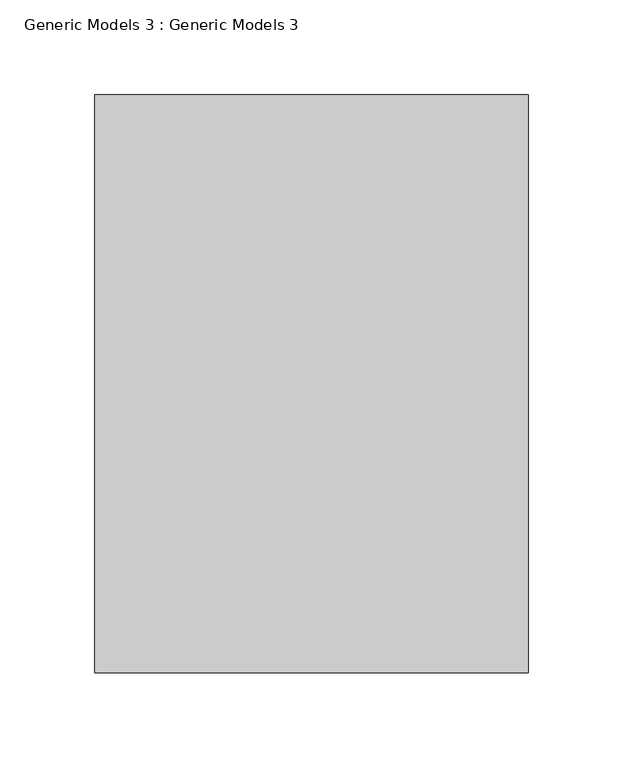
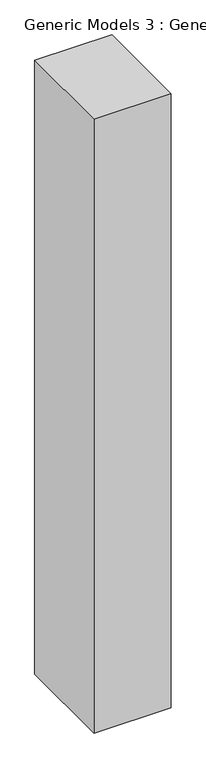
"""IFC4 building model written with IfcOpenShell, lengths in millimetres: proxy geometry, Generic Models 3 : Generic Models 3."""

from ifc_helpers import new_model, si_unit, frame, origin, place, context, project, spatial, polyline, outline, extrude, source, transform, mapped, element, save


def generic_models_3_generic_models_3_9be41323(model_context):
    return source(origin(), model_context, "Body", "SweptSolid", [
        extrude(outline(polyline([(-15608.868705, -5256.7027976), (-15380.268705, -5256.7027976), (-15380.268705, -5561.5027976), (-15608.868705, -5561.5027976), (-15608.868705, -5256.7027976)])), frame((0.0, 0.0, 457.2), z_axis=(0.0, 0.0, 1.0), x_axis=(1.0, 0.0, 0.0)), (0.0, 0.0, 1.0), 1922.2594115),
    ])


if __name__ == "__main__":
    model = new_model("IFC4")
    model_context = context("Model", 3, world=origin())
    ifc_project = project(units=[si_unit("LENGTHUNIT", "METRE", prefix="MILLI")], contexts=[model_context])
    site = spatial("IfcSite", under=ifc_project)
    building = spatial("IfcBuilding", under=site)
    placement = place(None, origin())
    generic_models_3_generic_models_3_shape = generic_models_3_generic_models_3_9be41323(model_context)
    element("IfcBuildingElementProxy", 1, Name="Generic Models 3 : Generic Models 3", ObjectType="Generic Models 3 : Generic Models 3", at=placement, inside=building, context=model_context, shape_type="MappedRepresentation", body=[
        mapped(generic_models_3_generic_models_3_shape, transform((0.0, 0.0, 0.0), x_axis=(1.0, 0.0, 0.0), y_axis=(0.0, 1.0, 0.0), z_axis=(0.0, 0.0, 1.0))),
    ])
    save(model, "model.ifc")
